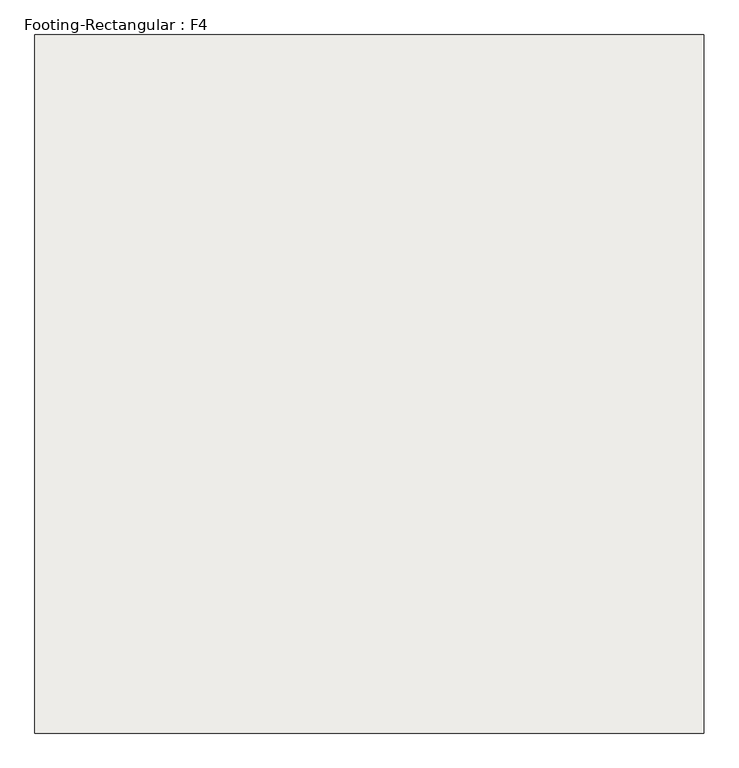
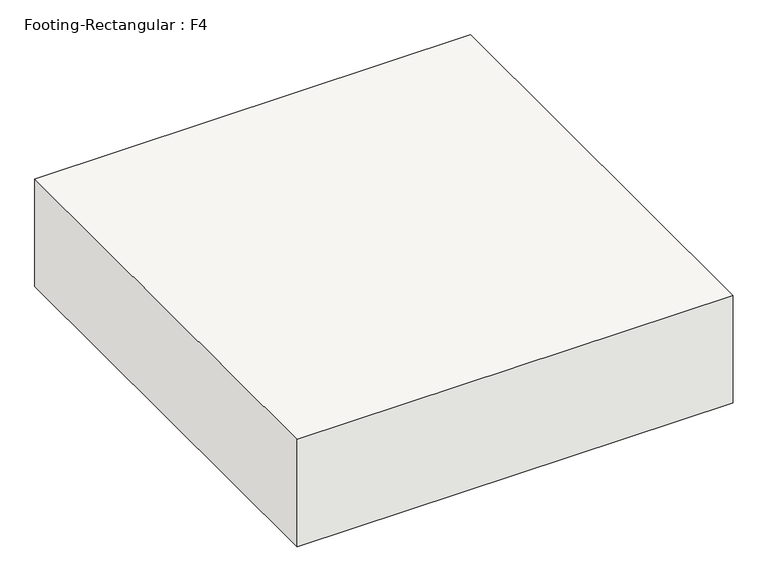
"""IFC4 building model written with IfcOpenShell, lengths in millimetres: slab geometry, Footing-Rectangular : F4."""

from ifc_helpers import new_model, si_unit, frame, origin, place, context, project, spatial, polyline, outline, extrude, source, transform, mapped, element, save


def footing_rectangular_f4_fcff0cd7(model_context):
    return source(origin(), model_context, "Body", "SweptSolid", [
        extrude(outline(polyline([(876.3, 914.4), (876.3, -914.4), (-876.3, -914.4), (-876.3, 914.4), (876.3, 914.4)])), frame((0.0, 0.0, -457.2), z_axis=(0.0, 0.0, 1.0), x_axis=(1.0, 0.0, 0.0)), (0.0, 0.0, 1.0), 457.2),
    ])


if __name__ == "__main__":
    model = new_model("IFC4")
    model_context = context("Model", 3, world=origin())
    ifc_project = project(units=[si_unit("LENGTHUNIT", "METRE", prefix="MILLI")], contexts=[model_context])
    site = spatial("IfcSite", under=ifc_project)
    building = spatial("IfcBuilding", under=site)
    placement = place(None, origin())
    footing_rectangular_f4_shape = footing_rectangular_f4_fcff0cd7(model_context)
    element("IfcSlab", 1, ObjectType="Footing-Rectangular : F4", at=placement, inside=building, context=model_context, shape_type="MappedRepresentation", body=[
        mapped(footing_rectangular_f4_shape, transform((0.0, 0.0, 0.0), x_axis=(1.0, 0.0, 0.0), y_axis=(0.0, 1.0, 0.0), z_axis=(0.0, 0.0, 1.0))),
    ])
    save(model, "model.ifc")

# Revit data of these elements
# Type "Footing-Rectangular : F4"
#   Width = 1752.6 mm
#   Length = 1828.8 mm
#   Foundation Thickness = 457.2 mm
#   Structural Material [instance default] = Concrete - Cast-in-Place Concrete
#   Assembly Code = ""
# Element 1 (IfcSlab, "Footing-Rectangular : F4")
#   Materials on its faces: "Concrete - Cast-in-Place Concrete"
# Materials
#   "Concrete - Cast-in-Place Concrete": class "Concrete", colour RGB 192 192 192, transparency 0, Cost = 0
